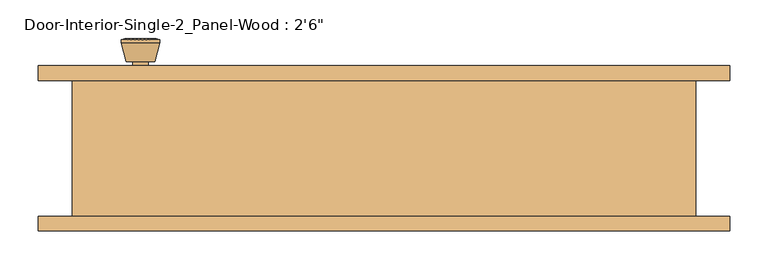
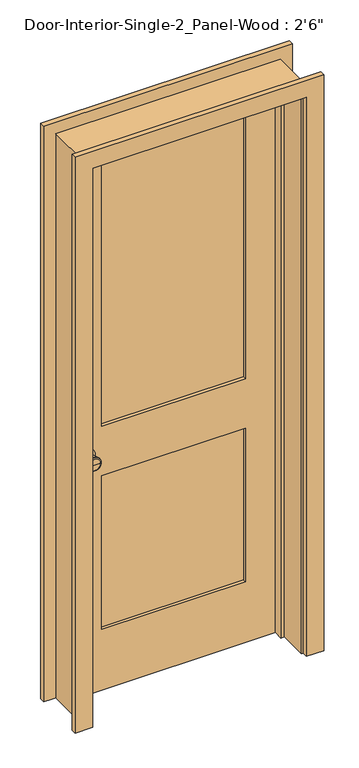
"""IFC4 building model written with IfcOpenShell, lengths in millimetres: door geometry."""

from ifc_helpers import new_model, si_unit, point, frame, frame_2d, origin, place, context, project, spatial, polyline, circle_curve, trimmed, segment, composite_curve, outline, extrude, faceted_brep, source, transform, mapped, element, save
from ifc_brep_helpers import plane_surface, cylinder_surface, revolved_surface, advanced_brep


def door_ff2e0a99(model_context):
    return source(origin(), model_context, "Body", "SolidModel", [
        advanced_brep(
        [(-317.5, 44.8, 914.4), (-307.5, 44.8, 914.4), (-327.5, 44.8, 914.4), (-297.0241324, -4.2, 914.4), (-317.5, -4.2, 914.4), (-337.9758676, -4.2, 914.4), (-292.5, -2.3721319, 914.4), (-342.5, -2.3721319, 914.4), (-292.5, 1.0915463, 914.4), (-342.5, 1.0915463, 914.4), (-298.863764, 25.8, 914.4), (-336.136236, 25.8, 914.4), (-307.5, 25.8, 914.4), (-327.5, 25.8, 914.4)],
        [
            (0, 1),
            (1, 2, circle_curve(frame((-317.5, 44.8, 914.4), z_axis=(0.0, 1.0, 0.0), x_axis=(-1.0, 0.0, 0.0)), 10.0)),
            (2, 0),
            (2, 1, circle_curve(frame((-317.5, 44.8, 914.4), z_axis=(0.0, 1.0, 0.0), x_axis=(-1.0, 0.0, 0.0)), 10.0)),
            (3, 4),
            (4, 5),
            (5, 3, circle_curve(frame((-317.5, -4.2, 914.4), z_axis=(0.0, -1.0, 0.0), x_axis=(-1.0, 0.0, 0.0)), 20.4758676)),
            (3, 5, circle_curve(frame((-317.5, -4.2, 914.4), z_axis=(0.0, -1.0, 0.0), x_axis=(-1.0, 0.0, 0.0)), 20.4758676)),
            (6, 3),
            (5, 7),
            (7, 6, circle_curve(frame((-317.5, -2.3721319, 914.4), z_axis=(0.0, -1.0, 0.0), x_axis=(-1.0, 0.0, 0.0)), 25.0)),
            (6, 7, circle_curve(frame((-317.5, -2.3721319, 914.4), z_axis=(0.0, -1.0, 0.0), x_axis=(-1.0, 0.0, 0.0)), 25.0)),
            (8, 6),
            (7, 9),
            (9, 8, circle_curve(frame((-317.5, 1.0915463, 914.4), z_axis=(0.0, -1.0, 0.0), x_axis=(-1.0, 0.0, 0.0)), 25.0)),
            (8, 9, circle_curve(frame((-317.5, 1.0915463, 914.4), z_axis=(0.0, -1.0, 0.0), x_axis=(-1.0, 0.0, 0.0)), 25.0)),
            (10, 8),
            (9, 11),
            (11, 10, circle_curve(frame((-317.5, 25.8, 914.4), z_axis=(0.0, -1.0, 0.0), x_axis=(-1.0, 0.0, 0.0)), 18.636236)),
            (10, 11, circle_curve(frame((-317.5, 25.8, 914.4), z_axis=(0.0, -1.0, 0.0), x_axis=(-1.0, 0.0, 0.0)), 18.636236)),
            (12, 10),
            (11, 13),
            (13, 12, circle_curve(frame((-317.5, 25.8, 914.4), z_axis=(0.0, -1.0, 0.0), x_axis=(-1.0, 0.0, 0.0)), 10.0)),
            (12, 13, circle_curve(frame((-317.5, 25.8, 914.4), z_axis=(0.0, -1.0, 0.0), x_axis=(-1.0, 0.0, 0.0)), 10.0)),
            (1, 12),
            (13, 2),
        ],
        [
            plane_surface(frame((-317.5, 44.8, 914.4), z_axis=(0.0, 1.0, 0.0), x_axis=(-1.0, 0.0, 0.0))),
            plane_surface(frame((-317.5, -4.2, 914.4), z_axis=(0.0, -1.0, 0.0), x_axis=(-1.0, 0.0, 0.0))),
            revolved_surface(polyline([(-337.9758676, -4.2, 914.4), (-342.5, -2.3721319, 914.4)]), (-317.5, 44.8, 914.4), (0.0, 1.0, 0.0)),
            cylinder_surface(frame((-317.5, 44.8, 914.4), z_axis=(0.0, 1.0, 0.0), x_axis=(-1.0, 0.0, 0.0)), 25.0),
            revolved_surface(polyline([(-342.5, 1.0915463, 914.4), (-336.136236, 25.8, 914.4)]), (-317.5, 44.8, 914.4), (0.0, 1.0, 0.0)),
            plane_surface(frame((-317.5, 25.8, 914.4), z_axis=(0.0, 1.0, 0.0), x_axis=(-1.0, 0.0, 0.0))),
            cylinder_surface(frame((-317.5, 44.8, 914.4), z_axis=(0.0, 1.0, 0.0), x_axis=(-1.0, 0.0, 0.0)), 10.0),
        ],
        [
            (0, [[1, 2, 3]]),
            (0, [[-3, 4, -1]]),
            (1, [[5, 6, 7]]),
            (1, [[-6, -5, 8]]),
            (2, [[9, -7, 10, 11]]),
            (2, [[-10, -8, -9, 12]]),
            (3, [[13, -11, 14, 15]]),
            (3, [[-14, -12, -13, 16]]),
            (4, [[17, -15, 18, 19]]),
            (4, [[-18, -16, -17, 20]]),
            (5, [[21, -19, 22, 23]]),
            (5, [[-22, -20, -21, 24]]),
            (6, [[25, -23, 26, -2]]),
            (6, [[-26, -24, -25, -4]]),
        ],
    ),
        extrude(outline(composite_curve([segment(trimmed(circle_curve(frame_2d((914.4, -317.5)), 30.0), [point((914.4, -347.5))], [point((914.4, -287.5))], False, "CARTESIAN"), True, "CONTINUOUS"), segment(trimmed(circle_curve(frame_2d((914.4, -317.5)), 30.0), [point((914.4, -287.5))], [point((914.4, -347.5))], False, "CARTESIAN"), True, "CONTINUOUS")], self_intersect=False)), frame((0.0, 44.8, 0.0), z_axis=(0.0, 1.0, 0.0), x_axis=(0.0, 0.0, 1.0)), (0.0, 0.0, 1.0), 6.0),
        advanced_brep(
        [(-317.5, 91.725, 914.4), (-327.5, 91.725, 914.4), (-307.5, 91.725, 914.4), (-297.0241324, 140.725, 914.4), (-337.9758676, 140.725, 914.4), (-317.5, 140.725, 914.4), (-292.5, 138.8971319, 914.4), (-342.5, 138.8971319, 914.4), (-292.5, 135.4334537, 914.4), (-342.5, 135.4334537, 914.4), (-298.863764, 110.725, 914.4), (-336.136236, 110.725, 914.4), (-307.5, 110.725, 914.4), (-327.5, 110.725, 914.4)],
        [
            (0, 1),
            (1, 2, circle_curve(frame((-317.5, 91.725, 914.4), z_axis=(0.0, -1.0, 0.0), x_axis=(-1.0, 0.0, 0.0)), 10.0)),
            (2, 0),
            (2, 1, circle_curve(frame((-317.5, 91.725, 914.4), z_axis=(0.0, -1.0, 0.0), x_axis=(-1.0, 0.0, 0.0)), 10.0)),
            (3, 4, circle_curve(frame((-317.5, 140.725, 914.4), z_axis=(0.0, 1.0, 0.0), x_axis=(-1.0, 0.0, 0.0)), 20.4758676)),
            (4, 5),
            (5, 3),
            (4, 3, circle_curve(frame((-317.5, 140.725, 914.4), z_axis=(0.0, 1.0, 0.0), x_axis=(-1.0, 0.0, 0.0)), 20.4758676)),
            (6, 7, circle_curve(frame((-317.5, 138.8971319, 914.4), z_axis=(0.0, 1.0, 0.0), x_axis=(-1.0, 0.0, 0.0)), 25.0)),
            (7, 4),
            (3, 6),
            (7, 6, circle_curve(frame((-317.5, 138.8971319, 914.4), z_axis=(0.0, 1.0, 0.0), x_axis=(-1.0, 0.0, 0.0)), 25.0)),
            (8, 9, circle_curve(frame((-317.5, 135.4334537, 914.4), z_axis=(0.0, 1.0, 0.0), x_axis=(-1.0, 0.0, 0.0)), 25.0)),
            (9, 7),
            (6, 8),
            (9, 8, circle_curve(frame((-317.5, 135.4334537, 914.4), z_axis=(0.0, 1.0, 0.0), x_axis=(-1.0, 0.0, 0.0)), 25.0)),
            (10, 11, circle_curve(frame((-317.5, 110.725, 914.4), z_axis=(0.0, 1.0, 0.0), x_axis=(-1.0, 0.0, 0.0)), 18.636236)),
            (11, 9),
            (8, 10),
            (11, 10, circle_curve(frame((-317.5, 110.725, 914.4), z_axis=(0.0, 1.0, 0.0), x_axis=(-1.0, 0.0, 0.0)), 18.636236)),
            (12, 13, circle_curve(frame((-317.5, 110.725, 914.4), z_axis=(0.0, 1.0, 0.0), x_axis=(-1.0, 0.0, 0.0)), 10.0)),
            (13, 11),
            (10, 12),
            (13, 12, circle_curve(frame((-317.5, 110.725, 914.4), z_axis=(0.0, 1.0, 0.0), x_axis=(-1.0, 0.0, 0.0)), 10.0)),
            (1, 13),
            (12, 2),
        ],
        [
            plane_surface(frame((-317.5, 91.725, 914.4), z_axis=(0.0, -1.0, 0.0), x_axis=(-1.0, 0.0, 0.0))),
            plane_surface(frame((-317.5, 140.725, 914.4), z_axis=(0.0, 1.0, 0.0), x_axis=(-1.0, 0.0, 0.0))),
            revolved_surface(polyline([(-337.9758676, 140.725, 914.4), (-342.5, 138.8971319, 914.4)]), (-317.5, 91.725, 914.4), (0.0, -1.0, 0.0)),
            cylinder_surface(frame((-317.5, 91.725, 914.4), z_axis=(0.0, -1.0, 0.0), x_axis=(-1.0, 0.0, 0.0)), 25.0),
            revolved_surface(polyline([(-342.5, 135.4334537, 914.4), (-336.136236, 110.725, 914.4)]), (-317.5, 91.725, 914.4), (0.0, -1.0, 0.0)),
            plane_surface(frame((-317.5, 110.725, 914.4), z_axis=(0.0, -1.0, 0.0), x_axis=(-1.0, 0.0, 0.0))),
            cylinder_surface(frame((-317.5, 91.725, 914.4), z_axis=(0.0, -1.0, 0.0), x_axis=(-1.0, 0.0, 0.0)), 10.0),
        ],
        [
            (0, [[1, 2, 3]]),
            (0, [[-3, 4, -1]]),
            (1, [[5, 6, 7]]),
            (1, [[8, -7, -6]]),
            (2, [[9, 10, -5, 11]]),
            (2, [[12, -11, -8, -10]]),
            (3, [[13, 14, -9, 15]]),
            (3, [[16, -15, -12, -14]]),
            (4, [[17, 18, -13, 19]]),
            (4, [[20, -19, -16, -18]]),
            (5, [[21, 22, -17, 23]]),
            (5, [[24, -23, -20, -22]]),
            (6, [[-2, 25, -21, 26]]),
            (6, [[-4, -26, -24, -25]]),
        ],
    ),
        extrude(outline(composite_curve([segment(trimmed(circle_curve(frame_2d((914.4, -317.5)), 30.0), [point((914.4, -347.5))], [point((914.4, -287.5))], False, "CARTESIAN"), True, "CONTINUOUS"), segment(trimmed(circle_curve(frame_2d((914.4, -317.5)), 30.0), [point((914.4, -287.5))], [point((914.4, -347.5))], False, "CARTESIAN"), True, "CONTINUOUS")], self_intersect=False)), frame((0.0, 85.725, 0.0), z_axis=(0.0, 1.0, 0.0), x_axis=(0.0, 0.0, 1.0)), (0.0, 0.0, 1.0), 6.0),
        faceted_brep([(406.4, 85.725, 0.0), (406.4, -92.075, 0.0), (381.0, -92.075, 0.0), (381.0, 15.875, 0.0), (368.3, 15.875, 0.0), (368.3, 50.8, 0.0), (381.0, 50.8, 0.0), (381.0, 85.725, 0.0), (406.4, 85.725, 2159.0), (406.4, -92.075, 2159.0), (-406.4, -92.075, 2159.0), (-406.4, -92.075, 0.0), (-381.0, -92.075, 0.0), (-381.0, -92.075, 2133.6), (381.0, -92.075, 2133.6), (381.0, 15.875, 2133.6), (-381.0, 15.875, 2133.6), (-381.0, 15.875, 0.0), (-368.3, 15.875, 0.0), (-368.3, 15.875, 2120.9), (368.3, 15.875, 2120.9), (368.3, 50.8, 2120.9), (-368.3, 50.8, 2120.9), (-368.3, 50.8, 0.0), (-381.0, 50.8, 0.0), (-381.0, 50.8, 2133.6), (381.0, 50.8, 2133.6), (381.0, 85.725, 2133.6), (-381.0, 85.725, 2133.6), (-381.0, 85.725, 0.0), (-406.4, 85.725, 0.0), (-406.4, 85.725, 2159.0)], [[[0, 1, 2, 3, 4, 5, 6, 7]], [[1, 0, 8, 9]], [[2, 1, 9, 10, 11, 12, 13, 14]], [[3, 2, 14, 15]], [[4, 3, 15, 16, 17, 18, 19, 20]], [[5, 4, 20, 21]], [[6, 5, 21, 22, 23, 24, 25, 26]], [[7, 6, 26, 27]], [[0, 7, 27, 28, 29, 30, 31, 8]], [[9, 8, 31, 10]], [[15, 14, 13, 16]], [[21, 20, 19, 22]], [[27, 26, 25, 28]], [[30, 29, 24, 23, 18, 17, 12, 11]], [[10, 31, 30, 11]], [[16, 13, 12, 17]], [[22, 19, 18, 23]], [[28, 25, 24, 29]]]),
        extrude(outline(polyline([(2133.6, -381.0), (0.0, -381.0), (0.0, 381.0), (2133.6, 381.0), (2133.6, -381.0)]), holes=[polyline([(2014.5375, -260.35), (2014.5375, 260.35), (1009.65, 260.35), (1009.65, -260.35), (2014.5375, -260.35)]), polyline([(819.15, -260.35), (819.15, 260.35), (231.775, 260.35), (231.775, -260.35), (819.15, -260.35)])]), frame((0.0, 50.8, 0.0), z_axis=(0.0, 1.0, 0.0), x_axis=(0.0, 0.0, 1.0)), (0.0, 0.0, 1.0), 34.925),
        extrude(outline(polyline([(260.35, 62.4416667), (-260.35, 62.4416667), (-260.35, 74.0833333), (260.35, 74.0833333), (260.35, 62.4416667)])), frame((0.0, 0.0, 1009.65), z_axis=(0.0, 0.0, 1.0), x_axis=(1.0, 0.0, 0.0)), (0.0, 0.0, 1.0), 1004.8875),
        extrude(outline(polyline([(260.35, 62.4416667), (-260.35, 62.4416667), (-260.35, 74.0833333), (260.35, 74.0833333), (260.35, 62.4416667)])), frame((0.0, 0.0, 231.775), z_axis=(0.0, 0.0, 1.0), x_axis=(1.0, 0.0, 0.0)), (0.0, 0.0, 1.0), 587.375),
        extrude(outline(polyline([(0.0, 387.35), (0.0, 450.85), (2203.45, 450.85), (2203.45, -450.85), (0.0, -450.85), (0.0, -387.35), (2139.95, -387.35), (2139.95, 387.35), (0.0, 387.35)])), frame((0.0, 85.725, 0.0), z_axis=(0.0, 1.0, 0.0), x_axis=(0.0, 0.0, 1.0)), (0.0, 0.0, 1.0), 19.05),
        extrude(outline(polyline([(0.0, 387.35), (0.0, 450.85), (2203.45, 450.85), (2203.45, -450.85), (0.0, -450.85), (0.0, -387.35), (2139.95, -387.35), (2139.95, 387.35), (0.0, 387.35)])), frame((0.0, -111.125, 0.0), z_axis=(0.0, 1.0, 0.0), x_axis=(0.0, 0.0, 1.0)), (0.0, 0.0, 1.0), 19.05),
    ])


if __name__ == "__main__":
    model = new_model("IFC4")
    model_context = context("Model", 3, world=origin())
    ifc_project = project(units=[si_unit("LENGTHUNIT", "METRE", prefix="MILLI")], contexts=[model_context])
    site = spatial("IfcSite", under=ifc_project)
    building = spatial("IfcBuilding", under=site)
    placement = place(None, origin())
    door_shape = door_ff2e0a99(model_context)
    element("IfcDoor", 1, ObjectType="Door-Interior-Single-2_Panel-Wood : 2'6\"", at=placement, inside=building, context=model_context, shape_type="MappedRepresentation", body=[
        mapped(door_shape, transform((0.0, 0.0, 0.0), x_axis=(1.0, 0.0, 0.0), y_axis=(0.0, 1.0, 0.0), z_axis=(0.0, 0.0, 1.0))),
    ])
    save(model, "model.ifc")

# Revit data of these elements
# Type "Door-Interior-Single-2_Panel-Wood : 2'6\""
#   Type Mark = "10"
#   Assembly Code = "C1020300"
#   Analytic Construction = "Wooden"
#   Top Rail = 0' - 4 11/16"
#   Thickness = 0' - 1 3/8"
#   Thermal Resistance (R) = 2.5876 (h·ft²·°F)/BTU
#   Swing Angle [instance default] = 90.00°
#   Stiles = 0' - 4 3/4"
#   Rough Width = 2' - 8"
#   Rough Height = 7' - 1"
#   Lock Rail = 0' - 7 1/2"
#   Height = 7' - 0"
#   Width = 2' - 6"
#   Heat Transfer Coefficient (U) = 0.3865 BTU/(h·ft²·°F)
#   Bottom Rail = 0' - 9 1/8"
#   Trim Material = Cherry
#   Panel Material = Cherry
#   Frame Material = Cherry
#   Door Handle Material = Aluminum
#   Visual Light Transmittance = 0
#   Solar Heat Gain Coefficient = 0
#   Wall Closure = (empty or 0)
#   Function = (empty or 0)
# Element 1 (IfcDoor, "Door-Interior-Single-2_Panel-Wood : 2'6\"")
#   Materials on its faces: "Cherry", "Aluminum"
# Materials
#   "Cherry": class "Wood", colour RGB 226 177 128, transparency 0, Description = "Prunus Serotina", Cost = 0
#   "Aluminum": class "Metal", colour RGB 247 247 247, transparency 0, Description = "Aluminum 6061", Cost = 0
